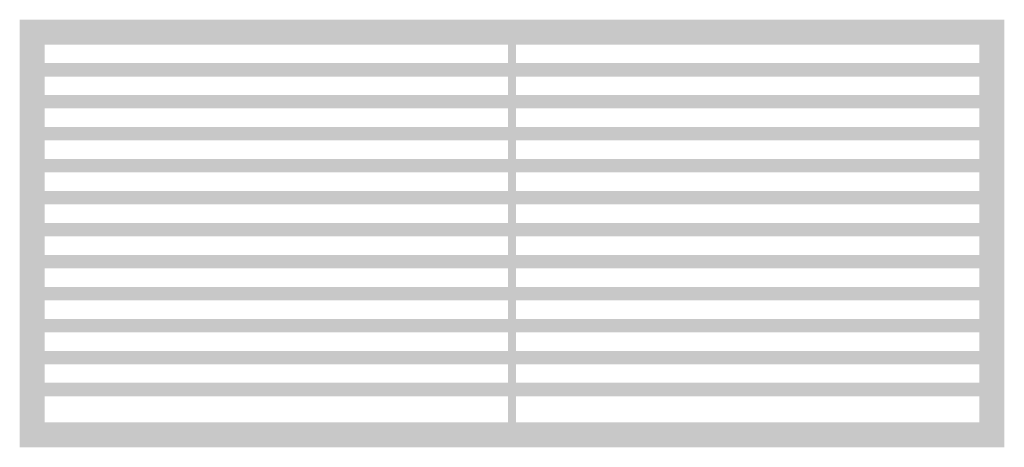
# Model space of a CAD drawing. Units: feet. Extents: x 2415 to 6174, y 866 to 1295.
# Tile 9 of 9: x 6015 to 6174, y 1018 to 1086. Entities that reach past the tile are written whole.
import ezdxf

# ---------------------------------------------------------------- set-up
doc = ezdxf.new("R2010")
doc.units = ezdxf.units.FT
doc.layers.add('A-ELEV-PATT', color=8, linetype='Continuous', lineweight=13)

msp = doc.modelspace()

# ---------------------------------------------------------------- hatches: boundary and pattern name
at = {"layer": 'A-ELEV-PATT'}
h = msp.add_hatch(color=256, dxfattribs=at)
h.set_gradient(color1=(147, 149, 152), color2=(99, 100, 102))
h.paths.add_polyline_path([(6173.9933, 1086.3639), (6015.3884, 1086.3639), (6015.3884, 1017.5301), (6173.9933, 1017.5301)])
h.paths.add_polyline_path([(6019.3884, 1082.3639), (6169.9933, 1082.3639), (6169.9933, 1021.5301), (6019.3884, 1021.5301)], flags=16)
h.paths.add_polyline_path([(6019.3884, 1079.3811), (6094.0601, 1079.3811), (6094.0601, 1082.3639), (6095.3216, 1082.3639), (6095.3216, 1079.3811), (6169.9933, 1079.3811), (6169.9933, 1077.2169), (6095.3216, 1077.2169), (6095.3216, 1074.2342), (6169.9933, 1074.2342), (6169.9933, 1072.07), (6095.3216, 1072.07), (6095.3216, 1069.0872), (6169.9933, 1069.0872), (6169.9933, 1066.923), (6095.3216, 1066.923), (6095.3216, 1063.9402), (6169.9933, 1063.9402), (6169.9933, 1061.7761), (6095.3216, 1061.7761), (6095.3216, 1058.7933), (6169.9933, 1058.7933), (6169.9933, 1056.6291), (6095.3216, 1056.6291), (6095.3216, 1053.6463), (6169.9933, 1053.6463), (6169.9933, 1051.4822), (6095.3216, 1051.4822), (6095.3216, 1048.4994), (6169.9933, 1048.4994), (6169.9933, 1046.3352), (6095.3216, 1046.3352), (6095.3216, 1043.3524), (6169.9933, 1043.3524), (6169.9933, 1041.1882), (6095.3216, 1041.1882), (6095.3216, 1038.2055), (6169.9933, 1038.2055), (6169.9933, 1036.0413), (6095.3216, 1036.0413), (6095.3216, 1033.0585), (6169.9933, 1033.0585), (6169.9933, 1030.8943), (6095.3216, 1030.8943), (6095.3216, 1027.9115), (6169.9933, 1027.9115), (6169.9933, 1025.7474), (6095.3216, 1025.7474), (6095.3216, 1021.5301), (6094.0601, 1021.5301), (6094.0601, 1025.7474), (6019.3884, 1025.7474), (6019.3884, 1027.9115), (6094.0601, 1027.9115), (6094.0601, 1030.8943), (6019.3884, 1030.8943), (6019.3884, 1033.0585), (6094.0601, 1033.0585), (6094.0601, 1036.0413), (6019.3884, 1036.0413), (6019.3884, 1038.2055), (6094.0601, 1038.2055), (6094.0601, 1041.1882), (6019.3884, 1041.1882), (6019.3884, 1043.3524), (6094.0601, 1043.3524), (6094.0601, 1046.3352), (6019.3884, 1046.3352), (6019.3884, 1048.4994), (6094.0601, 1048.4994), (6094.0601, 1051.4822), (6019.3884, 1051.4822), (6019.3884, 1053.6463), (6094.0601, 1053.6463), (6094.0601, 1056.6291), (6019.3884, 1056.6291), (6019.3884, 1058.7933), (6094.0601, 1058.7933), (6094.0601, 1061.7761), (6019.3884, 1061.7761), (6019.3884, 1063.9402), (6094.0601, 1063.9402), (6094.0601, 1066.923), (6019.3884, 1066.923), (6019.3884, 1069.0872), (6094.0601, 1069.0872), (6094.0601, 1072.07), (6019.3884, 1072.07), (6019.3884, 1074.2342), (6094.0601, 1074.2342), (6094.0601, 1077.2169), (6019.3884, 1077.2169)], flags=16)

doc.saveas('drawing.dxf')
